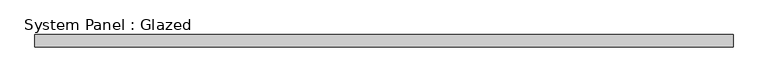
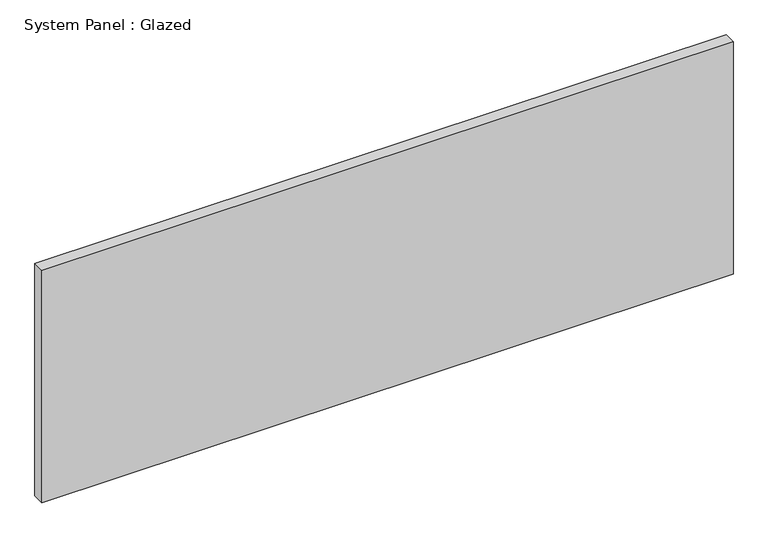
"""IFC4 building model written with IfcOpenShell, lengths in millimetres: plate geometry, System Panel : Glazed."""

from ifc_helpers import new_model, si_unit, origin, origin_with_axes, place, context, project, spatial, polyline, outline, extrude, source, transform, mapped, element, save


def system_panel_glazed_70a1cf78(model_context):
    return source(origin(), model_context, "Body", "SweptSolid", [
        extrude(outline(polyline([(723.4907433, -44.45), (-723.4907433, -44.45), (-723.4907433, -19.05), (723.4907433, -19.05), (723.4907433, -44.45)])), origin_with_axes(), (0.0, 0.0, 1.0), 514.35),
    ])


if __name__ == "__main__":
    model = new_model("IFC4")
    model_context = context("Model", 3, world=origin())
    ifc_project = project(units=[si_unit("LENGTHUNIT", "METRE", prefix="MILLI")], contexts=[model_context])
    site = spatial("IfcSite", under=ifc_project)
    building = spatial("IfcBuilding", under=site)
    placement = place(None, origin())
    system_panel_glazed_shape = system_panel_glazed_70a1cf78(model_context)
    element("IfcPlate", 1, ObjectType="System Panel : Glazed", at=placement, inside=building, context=model_context, shape_type="MappedRepresentation", body=[
        mapped(system_panel_glazed_shape, transform((0.0, 0.0, 0.0), x_axis=(1.0, 0.0, 0.0), y_axis=(0.0, 1.0, 0.0), z_axis=(0.0, 0.0, 1.0))),
    ])
    save(model, "model.ifc")

# Revit data of these elements
# Type "System Panel : Glazed"
#   Construction Type Id = "GSP4R"
#   Analytic Construction = "1/8 in Pilkington single glazing"
#   Visual Light Transmittance = 0.9
#   Solar Heat Gain Coefficient = 0.86
#   Heat Transfer Coefficient (U) = 1.18115 BTU/(h·ft²·°F)
# Element 1 (IfcPlate, "System Panel : Glazed")
#   Materials on its faces: "Glass"
# Materials
#   "Glass": class "Glass", colour RGB 0 128 192, transparency 0.75, Description = "Soda Lime Glass", Cost = 0
